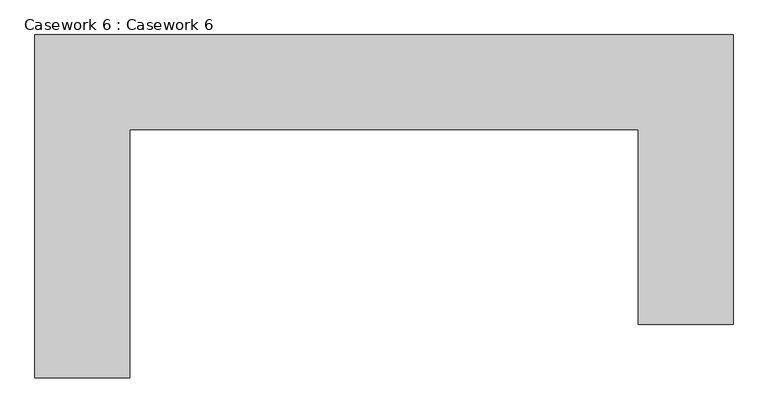
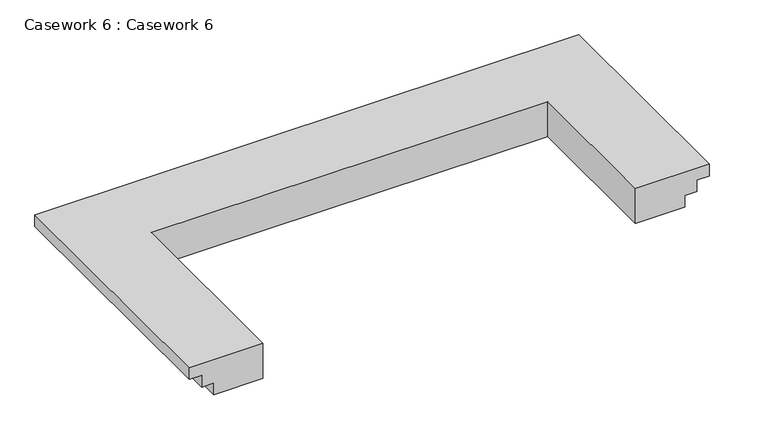
"""IFC4 building model written with IfcOpenShell, lengths in millimetres: furniture geometry, Casework 6 : Casework 6."""

from ifc_helpers import new_model, si_unit, origin, place, context, project, spatial, faceted_brep, source, transform, mapped, element, save


def casework_6_casework_6_bf376347(model_context):
    return source(origin(), model_context, "Body", "Brep", [
        faceted_brep([(3188.2046034, 8453.3070837, 4350.0), (3588.2046034, 8453.3070837, 4350.0), (3588.2046034, 8453.3070837, 4450.0), (3688.2046034, 8453.3070837, 4450.0), (3688.2046034, 8453.3070837, 4550.0), (3788.2046034, 8453.3070837, 4550.0), (3788.2046034, 8453.3070837, 4650.0), (3188.2046034, 8453.3070837, 4650.0), (3188.2046034, 9690.8070837, 4350.0), (-36.7953966, 9690.8070837, 4350.0), (-36.7953966, 8115.8070837, 4350.0), (-436.7953966, 8115.8070837, 4350.0), (-436.7953966, 10090.8070837, 4350.0), (3588.2046034, 10090.8070837, 4350.0), (3588.2046034, 10090.8070837, 4450.0), (-436.7953966, 10090.8070837, 4450.0), (-436.7953966, 8115.8070837, 4450.0), (-536.7953966, 8115.8070837, 4450.0), (-536.7953966, 10190.8070837, 4450.0), (3688.2046034, 10190.8070837, 4450.0), (3688.2046034, 10190.8070837, 4550.0), (-536.7953966, 10190.8070837, 4550.0), (-536.7953966, 8115.8070837, 4550.0), (-636.7953966, 8115.8070837, 4550.0), (-636.7953966, 10290.8070837, 4550.0), (3788.2046034, 10290.8070837, 4550.0), (3788.2046034, 10290.8070837, 4650.0), (-636.7953966, 10290.8070837, 4650.0), (-636.7953966, 8115.8070837, 4650.0), (-36.7953966, 8115.8070837, 4650.0), (-36.7953966, 9690.8070837, 4650.0), (3188.2046034, 9690.8070837, 4650.0)], [[[0, 1, 2, 3, 4, 5, 6, 7]], [[1, 0, 8, 9, 10, 11, 12, 13]], [[2, 1, 13, 14]], [[3, 2, 14, 15, 16, 17, 18, 19]], [[4, 3, 19, 20]], [[5, 4, 20, 21, 22, 23, 24, 25]], [[6, 5, 25, 26]], [[7, 6, 26, 27, 28, 29, 30, 31]], [[0, 7, 31, 8]], [[14, 13, 12, 15]], [[20, 19, 18, 21]], [[26, 25, 24, 27]], [[8, 31, 30, 9]], [[10, 29, 28, 23, 22, 17, 16, 11]], [[15, 12, 11, 16]], [[21, 18, 17, 22]], [[27, 24, 23, 28]], [[9, 30, 29, 10]]]),
    ])


if __name__ == "__main__":
    model = new_model("IFC4")
    model_context = context("Model", 3, world=origin())
    ifc_project = project(units=[si_unit("LENGTHUNIT", "METRE", prefix="MILLI")], contexts=[model_context])
    site = spatial("IfcSite", under=ifc_project)
    building = spatial("IfcBuilding", under=site)
    placement = place(None, origin())
    casework_6_casework_6_shape = casework_6_casework_6_bf376347(model_context)
    element("IfcFurniture", 1, ObjectType="Casework 6 : Casework 6", at=placement, inside=building, context=model_context, shape_type="MappedRepresentation", body=[
        mapped(casework_6_casework_6_shape, transform((0.0, 0.0, 0.0), x_axis=(1.0, 0.0, 0.0), y_axis=(0.0, 1.0, 0.0), z_axis=(0.0, 0.0, 1.0))),
    ])
    save(model, "model.ifc")
